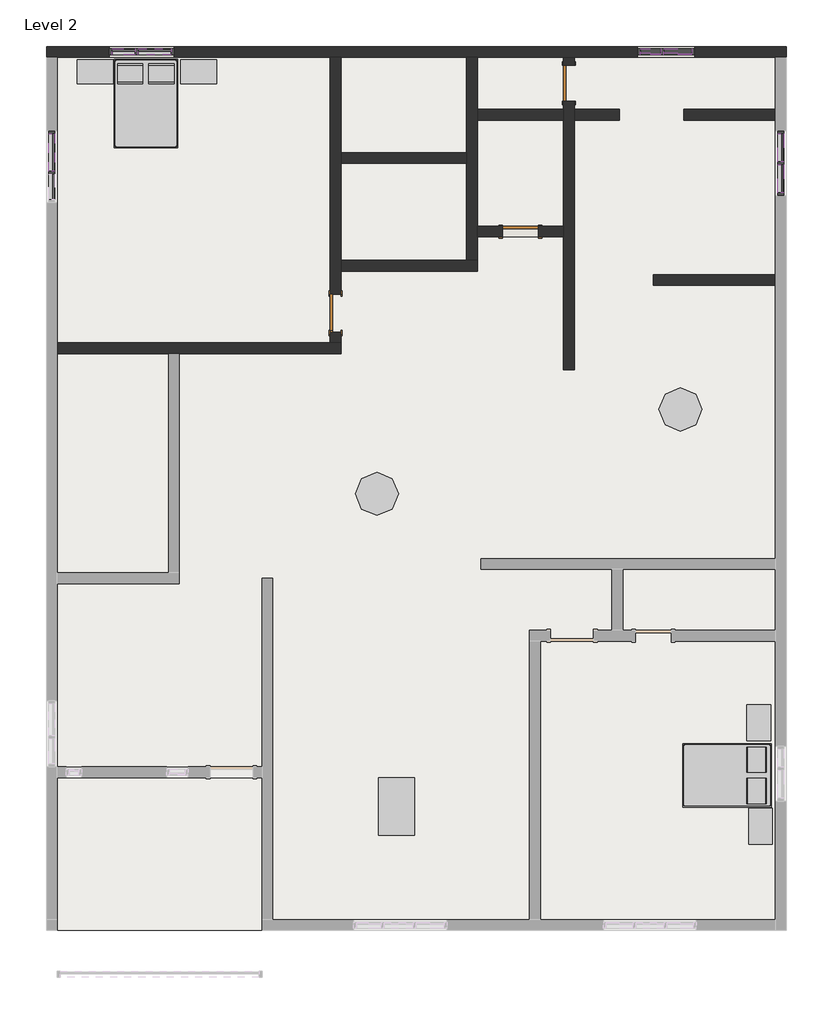
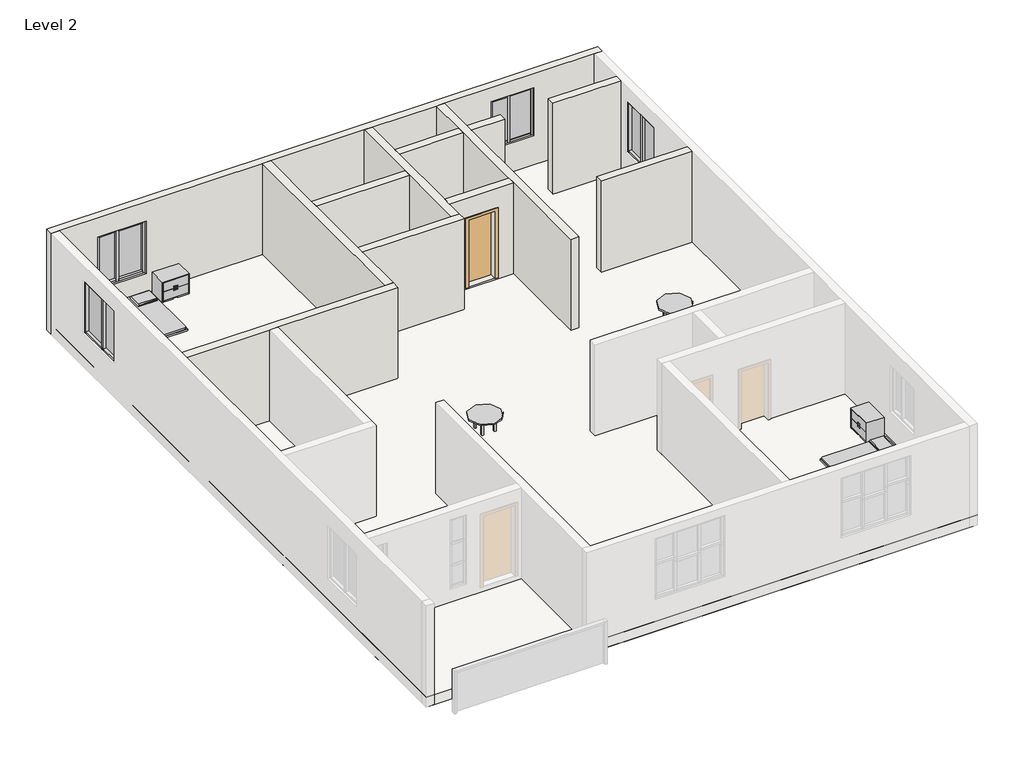
# One storey, part 3 of 3: 26 members, 12 walls, 9 furniture elements, 8 plates, 4 doors, 1 roof.
"""IFC4 building model written with IfcOpenShell, lengths in millimetres."""

from ifc_helpers import new_model, si_unit, frame, origin, place, context, project, spatial, polyline, outline, extrude, faceted_brep, transform, mapped, element, save
from components import door_a1484949, furniture_b58f7881, furniture_fb07e05e, furniture_acc2807d, furniture_52f35bf4, member_b9f3750b, member_5f1d7e17, member_e5d39754, member_104ec00a, member_3b277a63, member_6fb4a552, member_a4862887, member_e55e8fcb, member_9145ce8f, member_65d07e0b, member_13dc6413, member_cb82b20f, member_81de2198, member_b315899a, system_panel_glazed_d0271aee, system_panel_glazed_77db913b, system_panel_glazed_12bad0c7, system_panel_glazed_328f5a3b, system_panel_glazed_ae4b356e, system_panel_glazed_89fef50d, system_panel_glazed_cb6b9410

model = new_model("IFC4")

# Units and contexts
model_context = context("Model", 3, world=origin())
ifc_project = project(units=[si_unit("LENGTHUNIT", "METRE", prefix="MILLI")], contexts=[model_context])

# Site, building, storey
site = spatial("IfcSite", under=ifc_project)
building = spatial("IfcBuilding", under=site)
storey = spatial("IfcBuildingStorey", under=building, Name="Level 2", Elevation=3048.0)

# Doors
placement = place(None, origin())
door_shape = door_a1484949(model_context)
element("IfcDoor", 1, ObjectType="Single-Flush : 30\" x 80\"", at=placement, inside=storey, context=model_context, shape_type="MappedRepresentation", body=[
    mapped(door_shape, transform((-12951.6702714, 1518.6616097, 3048.0), x_axis=(0.0, 1.0, 0.0), y_axis=(-1.0, 0.0, 0.0), z_axis=(0.0, 0.0, 1.0))),
])
element("IfcDoor", 2, ObjectType="Single-Flush : 30\" x 80\"", at=placement, inside=storey, context=model_context, shape_type="MappedRepresentation", body=[
    mapped(door_shape, transform((-12951.6702714, 1480.5616097, 3048.0), x_axis=(0.0, 1.0, 0.0), y_axis=(-1.0, 0.0, 0.0), z_axis=(0.0, 0.0, 1.0))),
])
element("IfcDoor", 3, ObjectType="Single-Flush : 30\" x 80\"", at=placement, inside=storey, context=model_context, shape_type="MappedRepresentation", body=[
    mapped(door_shape, transform((-9027.3702714, 3233.1616097, 3403.6), x_axis=(1.0, 0.0, 0.0), y_axis=(0.0, 1.0, 0.0), z_axis=(0.0, 0.0, 1.0))),
])
element("IfcDoor", 4, ObjectType="Single-Flush : 30\" x 80\"", at=placement, inside=storey, context=model_context, shape_type="MappedRepresentation", body=[
    mapped(door_shape, transform((-7998.6702714, 6376.4116097, 3048.0), x_axis=(0.0, 1.0, 0.0), y_axis=(-1.0, 0.0, 0.0), z_axis=(0.0, 0.0, 1.0))),
])

# Furniture
furniture_shape = furniture_b58f7881(model_context)
element("IfcFurniture", 5, ObjectType="Bed-Box : Double 53\" x 74\"", at=placement, inside=storey, context=model_context, shape_type="MappedRepresentation", body=[
    mapped(furniture_shape, transform((-17316.7227304, 6185.3911179, 3048.0), x_axis=(1.0, 0.0, 0.0), y_axis=(0.0, 1.0, 0.0), z_axis=(0.0, 0.0, 1.0))),
])
element("IfcFurniture", 6, ObjectType="Bed-Box : Double 53\" x 74\"", at=placement, inside=storey, context=model_context, shape_type="MappedRepresentation", body=[
    mapped(furniture_shape, transform((-4411.4407632, -7959.2859313, 3048.0), x_axis=(0.0, -1.0, 0.0), y_axis=(1.0, 0.0, 0.0), z_axis=(0.0, 0.0, 1.0))),
])
furniture_2_shape = furniture_fb07e05e(model_context)
element("IfcFurniture", 7, ObjectType="Cabinet File-Lateral 3 Drawer : 30\" x 20\" x 36\"", at=placement, inside=storey, context=model_context, shape_type="MappedRepresentation", body=[
    mapped(furniture_2_shape, transform((-15679.9477575, 7558.3799858, 3048.0), x_axis=(1.0, 0.0, 0.0), y_axis=(0.0, 1.0, 0.0), z_axis=(0.0, 0.0, 1.0))),
])
element("IfcFurniture", 8, ObjectType="Cabinet File-Lateral 3 Drawer : 30\" x 20\" x 36\"", at=placement, inside=storey, context=model_context, shape_type="MappedRepresentation", body=[
    mapped(furniture_2_shape, transform((-17877.0477575, 7558.3799858, 3048.0), x_axis=(1.0, 0.0, 0.0), y_axis=(0.0, 1.0, 0.0), z_axis=(0.0, 0.0, 1.0))),
])
element("IfcFurniture", 9, ObjectType="Cabinet File-Lateral 3 Drawer : 30\" x 20\" x 36\"", at=placement, inside=storey, context=model_context, shape_type="MappedRepresentation", body=[
    mapped(furniture_2_shape, transform((-3038.4518953, -7360.8609042, 3048.0), x_axis=(0.0, -1.0, 0.0), y_axis=(1.0, 0.0, 0.0), z_axis=(0.0, 0.0, 1.0))),
])
element("IfcFurniture", 10, ObjectType="Cabinet File-Lateral 3 Drawer : 30\" x 20\" x 36\"", at=placement, inside=storey, context=model_context, shape_type="MappedRepresentation", body=[
    mapped(furniture_2_shape, transform((-3000.3518953, -9557.9609042, 3048.0), x_axis=(0.0, -1.0, 0.0), y_axis=(1.0, 0.0, 0.0), z_axis=(0.0, 0.0, 1.0))),
])
furniture_3_shape = furniture_acc2807d(model_context)
element("IfcFurniture", 11, ObjectType="Table-Coffee Rectangular : 48\" x 30\"", at=placement, inside=storey, context=model_context, shape_type="MappedRepresentation", body=[
    mapped(furniture_3_shape, transform((-11286.6594396, -9572.1720206, 3048.0), x_axis=(0.0, 1.0, 0.0), y_axis=(-1.0, 0.0, 0.0), z_axis=(0.0, 0.0, 1.0))),
])
furniture_4_shape = furniture_52f35bf4(model_context)
element("IfcFurniture", 12, ObjectType="Table-Dining Round w Chairs : 36\" Diameter", at=placement, inside=storey, context=model_context, shape_type="MappedRepresentation", body=[
    mapped(furniture_4_shape, transform((-5740.1522386, -353.8597018, 3048.0), x_axis=(1.0, 0.0, 0.0), y_axis=(0.0, 1.0, 0.0), z_axis=(0.0, 0.0, 1.0))),
])
element("IfcFurniture", 13, ObjectType="Table-Dining Round w Chairs : 36\" Diameter", at=placement, inside=storey, context=model_context, shape_type="MappedRepresentation", body=[
    mapped(furniture_4_shape, transform((-12179.0522386, -2144.5597018, 3048.0), x_axis=(1.0, 0.0, 0.0), y_axis=(0.0, 1.0, 0.0), z_axis=(0.0, 0.0, 1.0))),
])

# Members
member_shape = member_b9f3750b(model_context)
element("IfcMember", 14, ObjectType="Rectangular Mullion : 2.5\" x 5\" rectangular", at=placement, inside=storey, context=model_context, shape_type="MappedRepresentation", body=[
    mapped(member_shape, transform((-17688.7702714, 7043.1616097, 3942.1035042), x_axis=(0.0, 0.0, -1.0), y_axis=(0.0, -1.0, 0.0), z_axis=(-1.0, 0.0, 0.0))),
])
element("IfcMember", 15, ObjectType="Rectangular Mullion : 2.5\" x 5\" rectangular", at=placement, inside=storey, context=model_context, shape_type="MappedRepresentation", body=[
    mapped(member_shape, transform((-17199.8202714, 7043.1616097, 5518.94108), x_axis=(0.0, 0.0, 1.0), y_axis=(0.0, -1.0, 0.0), z_axis=(1.0, 0.0, 0.0))),
])
member_2_shape = member_5f1d7e17(model_context)
element("IfcMember", 16, ObjectType="Rectangular Mullion : 2.5\" x 5\" rectangular", at=placement, inside=storey, context=model_context, shape_type="MappedRepresentation", body=[
    mapped(member_2_shape, transform((-16444.1702714, 7043.1616097, 5518.94108), x_axis=(0.0, 0.0, 1.0), y_axis=(0.0, -1.0, 0.0), z_axis=(1.0, 0.0, 0.0))),
])
element("IfcMember", 17, ObjectType="Rectangular Mullion : 2.5\" x 5\" rectangular", at=placement, inside=storey, context=model_context, shape_type="MappedRepresentation", body=[
    mapped(member_2_shape, transform((-17136.3202714, 7043.1616097, 3942.1035042), x_axis=(0.0, 0.0, -1.0), y_axis=(0.0, -1.0, 0.0), z_axis=(-1.0, 0.0, 0.0))),
])
member_3_shape = member_e5d39754(model_context)
element("IfcMember", 18, ObjectType="Rectangular Mullion : 2.5\" x 5\" rectangular", at=placement, inside=storey, context=model_context, shape_type="MappedRepresentation", body=[
    mapped(member_3_shape, transform((-3502.8702714, 4712.7116097, 5644.9656178), x_axis=(0.0, 0.0, 1.0), y_axis=(-1.0, 0.0, 0.0), z_axis=(0.0, -1.0, 0.0))),
])
element("IfcMember", 19, ObjectType="Rectangular Mullion : 2.5\" x 5\" rectangular", at=placement, inside=storey, context=model_context, shape_type="MappedRepresentation", body=[
    mapped(member_3_shape, transform((-3502.8702714, 4058.6616097, 5644.9656178), x_axis=(0.0, 0.0, 1.0), y_axis=(-1.0, 0.0, 0.0), z_axis=(0.0, -1.0, 0.0))),
])
element("IfcMember", 20, ObjectType="Rectangular Mullion : 2.5\" x 5\" rectangular", at=placement, inside=storey, context=model_context, shape_type="MappedRepresentation", body=[
    mapped(member_3_shape, transform((-5985.7202714, 7043.1616097, 5678.8107685), x_axis=(0.0, 0.0, 1.0), y_axis=(0.0, 1.0, 0.0), z_axis=(-1.0, 0.0, 0.0))),
])
element("IfcMember", 21, ObjectType="Rectangular Mullion : 2.5\" x 5\" rectangular", at=placement, inside=storey, context=model_context, shape_type="MappedRepresentation", body=[
    mapped(member_3_shape, transform((-3502.8702714, 4649.2116097, 4078.2335743), x_axis=(0.0, 0.0, -1.0), y_axis=(-1.0, 0.0, 0.0), z_axis=(0.0, 1.0, 0.0))),
])
element("IfcMember", 22, ObjectType="Rectangular Mullion : 2.5\" x 5\" rectangular", at=placement, inside=storey, context=model_context, shape_type="MappedRepresentation", body=[
    mapped(member_3_shape, transform((-3502.8702714, 5303.2616097, 4078.2335743), x_axis=(0.0, 0.0, -1.0), y_axis=(-1.0, 0.0, 0.0), z_axis=(0.0, 1.0, 0.0))),
])
element("IfcMember", 23, ObjectType="Rectangular Mullion : 2.5\" x 5\" rectangular", at=placement, inside=storey, context=model_context, shape_type="MappedRepresentation", body=[
    mapped(member_3_shape, transform((-5395.1702714, 7043.1616097, 4231.7599798), x_axis=(0.0, 0.0, -1.0), y_axis=(0.0, 1.0, 0.0), z_axis=(1.0, 0.0, 0.0))),
])
member_4_shape = member_104ec00a(model_context)
element("IfcMember", 24, ObjectType="Rectangular Mullion : 2.5\" x 5\" rectangular", at=placement, inside=storey, context=model_context, shape_type="MappedRepresentation", body=[
    mapped(member_4_shape, transform((-3502.8702714, 4680.9616097, 4078.2335743), x_axis=(0.0, -1.0, 0.0), y_axis=(-1.0, 0.0, 0.0), z_axis=(0.0, 0.0, -1.0))),
])
member_5_shape = member_3b277a63(model_context)
element("IfcMember", 25, ObjectType="Rectangular Mullion : 2.5\" x 5\" rectangular", at=placement, inside=storey, context=model_context, shape_type="MappedRepresentation", body=[
    mapped(member_5_shape, transform((-3502.8702714, 5366.7616097, 5644.9656178), x_axis=(0.0, 1.0, 0.0), y_axis=(-1.0, 0.0, 0.0), z_axis=(0.0, 0.0, 1.0))),
])
element("IfcMember", 26, ObjectType="Rectangular Mullion : 2.5\" x 5\" rectangular", at=placement, inside=storey, context=model_context, shape_type="MappedRepresentation", body=[
    mapped(member_5_shape, transform((-3502.8702714, 3995.1616097, 4078.2335743), x_axis=(0.0, -1.0, 0.0), y_axis=(-1.0, 0.0, 0.0), z_axis=(0.0, 0.0, -1.0))),
])
member_6_shape = member_6fb4a552(model_context)
element("IfcMember", 27, ObjectType="Rectangular Mullion : 2.5\" x 5\" rectangular", at=placement, inside=storey, context=model_context, shape_type="MappedRepresentation", body=[
    mapped(member_6_shape, transform((-6487.3702714, 7043.1616097, 5678.8107685), x_axis=(0.0, 0.0, 1.0), y_axis=(0.0, 1.0, 0.0), z_axis=(-1.0, 0.0, 0.0))),
])
member_7_shape = member_a4862887(model_context)
element("IfcMember", 28, ObjectType="Rectangular Mullion : 2.5\" x 5\" rectangular", at=placement, inside=storey, context=model_context, shape_type="MappedRepresentation", body=[
    mapped(member_7_shape, transform((-6017.4702714, 7043.1616097, 4231.7599798), x_axis=(-1.0, 0.0, 0.0), y_axis=(0.0, 1.0, 0.0), z_axis=(0.0, 0.0, -1.0))),
])
element("IfcMember", 29, ObjectType="Rectangular Mullion : 2.5\" x 5\" rectangular", at=placement, inside=storey, context=model_context, shape_type="MappedRepresentation", body=[
    mapped(member_6_shape, transform((-6049.2202714, 7043.1616097, 4231.7599798), x_axis=(0.0, 0.0, -1.0), y_axis=(0.0, 1.0, 0.0), z_axis=(1.0, 0.0, 0.0))),
])
member_8_shape = member_e55e8fcb(model_context)
element("IfcMember", 30, ObjectType="Rectangular Mullion : 2.5\" x 5\" rectangular", at=placement, inside=storey, context=model_context, shape_type="MappedRepresentation", body=[
    mapped(member_8_shape, transform((-6550.8702714, 7043.1616097, 4231.7599798), x_axis=(-1.0, 0.0, 0.0), y_axis=(0.0, 1.0, 0.0), z_axis=(0.0, 0.0, -1.0))),
])
element("IfcMember", 31, ObjectType="Rectangular Mullion : 2.5\" x 5\" rectangular", at=placement, inside=storey, context=model_context, shape_type="MappedRepresentation", body=[
    mapped(member_8_shape, transform((-5331.6702714, 7043.1616097, 5678.8107685), x_axis=(1.0, 0.0, 0.0), y_axis=(0.0, 1.0, 0.0), z_axis=(0.0, 0.0, 1.0))),
])
member_9_shape = member_9145ce8f(model_context)
element("IfcMember", 32, ObjectType="Rectangular Mullion : 2.5\" x 5\" rectangular", at=placement, inside=storey, context=model_context, shape_type="MappedRepresentation", body=[
    mapped(member_9_shape, transform((-17168.0702714, 7043.1616097, 3942.1035042), x_axis=(1.0, 0.0, 0.0), y_axis=(0.0, -1.0, 0.0), z_axis=(0.0, 0.0, -1.0))),
])
member_10_shape = member_65d07e0b(model_context)
element("IfcMember", 33, ObjectType="Rectangular Mullion : 2.5\" x 5\" rectangular", at=placement, inside=storey, context=model_context, shape_type="MappedRepresentation", body=[
    mapped(member_10_shape, transform((-17752.2702714, 7043.1616097, 5518.94108), x_axis=(-1.0, 0.0, 0.0), y_axis=(0.0, -1.0, 0.0), z_axis=(0.0, 0.0, 1.0))),
])
element("IfcMember", 34, ObjectType="Rectangular Mullion : 2.5\" x 5\" rectangular", at=placement, inside=storey, context=model_context, shape_type="MappedRepresentation", body=[
    mapped(member_10_shape, transform((-16380.6702714, 7043.1616097, 3942.1035042), x_axis=(1.0, 0.0, 0.0), y_axis=(0.0, -1.0, 0.0), z_axis=(0.0, 0.0, -1.0))),
])
member_11_shape = member_13dc6413(model_context)
element("IfcMember", 35, ObjectType="Rectangular Mullion : 2.5\" x 5\" rectangular", at=placement, inside=storey, context=model_context, shape_type="MappedRepresentation", body=[
    mapped(member_11_shape, transform((-18971.4702714, 4509.5116097, 5636.3811186), x_axis=(0.0, 0.0, 1.0), y_axis=(-1.0, 0.0, 0.0), z_axis=(0.0, -1.0, 0.0))),
])
member_12_shape = member_cb82b20f(model_context)
element("IfcMember", 36, ObjectType="Rectangular Mullion : 2.5\" x 5\" rectangular", at=placement, inside=storey, context=model_context, shape_type="MappedRepresentation", body=[
    mapped(member_12_shape, transform((-18971.4702714, 4477.7616097, 4041.7365925), x_axis=(0.0, -1.0, 0.0), y_axis=(-1.0, 0.0, 0.0), z_axis=(0.0, 0.0, -1.0))),
])
member_13_shape = member_81de2198(model_context)
element("IfcMember", 37, ObjectType="Rectangular Mullion : 2.5\" x 5\" rectangular", at=placement, inside=storey, context=model_context, shape_type="MappedRepresentation", body=[
    mapped(member_13_shape, transform((-18971.4702714, 4446.0116097, 4041.7365925), x_axis=(0.0, 0.0, -1.0), y_axis=(-1.0, 0.0, 0.0), z_axis=(0.0, 1.0, 0.0))),
])
element("IfcMember", 38, ObjectType="Rectangular Mullion : 2.5\" x 5\" rectangular", at=placement, inside=storey, context=model_context, shape_type="MappedRepresentation", body=[
    mapped(member_11_shape, transform((-18971.4702714, 5303.2616097, 4041.7365925), x_axis=(0.0, 0.0, -1.0), y_axis=(-1.0, 0.0, 0.0), z_axis=(0.0, 1.0, 0.0))),
])
member_14_shape = member_b315899a(model_context)
element("IfcMember", 39, ObjectType="Rectangular Mullion : 2.5\" x 5\" rectangular", at=placement, inside=storey, context=model_context, shape_type="MappedRepresentation", body=[
    mapped(member_14_shape, transform((-18971.4702714, 5366.7616097, 5636.3811186), x_axis=(0.0, 1.0, 0.0), y_axis=(-1.0, 0.0, 0.0), z_axis=(0.0, 0.0, 1.0))),
])

# Plates
system_panel_glazed_shape = system_panel_glazed_d0271aee(model_context)
element("IfcPlate", 40, ObjectType="System Panel : Glazed", at=placement, inside=storey, context=model_context, shape_type="MappedRepresentation", body=[
    mapped(system_panel_glazed_shape, transform((-3502.8702714, 5007.9866097, 4141.7335743), x_axis=(0.0, -1.0, 0.0), y_axis=(1.0, 0.0, 0.0), z_axis=(0.0, 0.0, 1.0))),
])
element("IfcPlate", 41, ObjectType="System Panel : Glazed", at=placement, inside=storey, context=model_context, shape_type="MappedRepresentation", body=[
    mapped(system_panel_glazed_shape, transform((-3502.8702714, 4353.9366097, 4141.7335743), x_axis=(0.0, -1.0, 0.0), y_axis=(1.0, 0.0, 0.0), z_axis=(0.0, 0.0, 1.0))),
])
system_panel_glazed_2_shape = system_panel_glazed_77db913b(model_context)
element("IfcPlate", 42, ObjectType="System Panel : Glazed", at=placement, inside=storey, context=model_context, shape_type="MappedRepresentation", body=[
    mapped(system_panel_glazed_2_shape, transform((-5690.4452714, 7043.1616097, 4295.2599798), x_axis=(-1.0, 0.0, 0.0), y_axis=(0.0, -1.0, 0.0), z_axis=(0.0, 0.0, 1.0))),
])
system_panel_glazed_3_shape = system_panel_glazed_12bad0c7(model_context)
element("IfcPlate", 43, ObjectType="System Panel : Glazed", at=placement, inside=storey, context=model_context, shape_type="MappedRepresentation", body=[
    mapped(system_panel_glazed_3_shape, transform((-6268.2952714, 7043.1616097, 4295.2599798), x_axis=(-1.0, 0.0, 0.0), y_axis=(0.0, -1.0, 0.0), z_axis=(0.0, 0.0, 1.0))),
])
system_panel_glazed_4_shape = system_panel_glazed_328f5a3b(model_context)
element("IfcPlate", 44, ObjectType="System Panel : Glazed", at=placement, inside=storey, context=model_context, shape_type="MappedRepresentation", body=[
    mapped(system_panel_glazed_4_shape, transform((-17444.2952714, 7043.1616097, 4005.6035042), x_axis=(1.0, 0.0, 0.0), y_axis=(0.0, 1.0, 0.0), z_axis=(0.0, 0.0, 1.0))),
])
system_panel_glazed_5_shape = system_panel_glazed_ae4b356e(model_context)
element("IfcPlate", 45, ObjectType="System Panel : Glazed", at=placement, inside=storey, context=model_context, shape_type="MappedRepresentation", body=[
    mapped(system_panel_glazed_5_shape, transform((-16790.2452714, 7043.1616097, 4005.6035042), x_axis=(1.0, 0.0, 0.0), y_axis=(0.0, 1.0, 0.0), z_axis=(0.0, 0.0, 1.0))),
])
system_panel_glazed_6_shape = system_panel_glazed_89fef50d(model_context)
element("IfcPlate", 46, ObjectType="System Panel : Glazed", at=placement, inside=storey, context=model_context, shape_type="MappedRepresentation", body=[
    mapped(system_panel_glazed_6_shape, transform((-18971.4702714, 4906.3866097, 4105.2365925), x_axis=(0.0, -1.0, 0.0), y_axis=(1.0, 0.0, 0.0), z_axis=(0.0, 0.0, 1.0))),
])
system_panel_glazed_7_shape = system_panel_glazed_cb6b9410(model_context)
element("IfcPlate", 47, ObjectType="System Panel : Glazed", at=placement, inside=storey, context=model_context, shape_type="MappedRepresentation", body=[
    mapped(system_panel_glazed_7_shape, transform((-18971.4702714, 4176.1366097, 4105.2365925), x_axis=(0.0, -1.0, 0.0), y_axis=(1.0, 0.0, 0.0), z_axis=(0.0, 0.0, 1.0))),
])

# Roof
element("IfcRoof", 48, ObjectType="Generic - 12\"", at=placement, inside=storey, context=model_context, shape_type="SweptSolid", body=[
    extrude(outline(polyline([(-19085.7702714, 7157.4616097), (-3388.5702714, 7157.4616097), (-3388.5702714, -11587.7383903), (-19085.7702714, -11587.7383903), (-19085.7702714, 7157.4616097)])), frame((0.0, 0.0, 3048.0), z_axis=(0.0, 0.0, 1.0), x_axis=(1.0, 0.0, 0.0)), (0.0, 0.0, 1.0), 304.8),
])

# Walls
element("IfcWall", 49, ObjectType="9\"", at=placement, inside=storey, context=model_context, shape_type="Brep", body=[
    faceted_brep([(-19085.7702714, 6928.8616097, 3048.0), (-18857.1702714, 6928.8616097, 3048.0), (-13065.9702714, 6928.8616097, 3048.0), (-12837.3702714, 6928.8616097, 3048.0), (-10170.3702714, 6928.8616097, 3048.0), (-9941.7702714, 6928.8616097, 3048.0), (-8112.9702714, 6928.8616097, 3048.0), (-7884.3702714, 6928.8616097, 3048.0), (-3617.1702714, 6928.8616097, 3048.0), (-3388.5702714, 6928.8616097, 3048.0), (-3388.5702714, 6928.8616097, 6096.0), (-3617.1702714, 6928.8616097, 6096.0), (-7884.3702714, 6928.8616097, 6096.0), (-8112.9702714, 6928.8616097, 6096.0), (-9941.7702714, 6928.8616097, 6096.0), (-10170.3702714, 6928.8616097, 6096.0), (-12837.3702714, 6928.8616097, 6096.0), (-13065.9702714, 6928.8616097, 6096.0), (-18857.1702714, 6928.8616097, 6096.0), (-19085.7702714, 6928.8616097, 6096.0), (-5331.6702714, 6928.8616097, 5678.8107685), (-5331.6702714, 6928.8616097, 4231.7599798), (-6550.8702714, 6928.8616097, 4231.7599798), (-6550.8702714, 6928.8616097, 5678.8107685), (-17752.2702714, 6928.8616097, 3942.1035042), (-17752.2702714, 6928.8616097, 5518.94108), (-16380.6702714, 6928.8616097, 5518.94108), (-16380.6702714, 6928.8616097, 3942.1035042), (-3388.5702714, 7157.4616097, 3048.0), (-19085.7702714, 7157.4616097, 3048.0), (-19085.7702714, 7157.4616097, 6096.0), (-3388.5702714, 7157.4616097, 6096.0), (-5331.6702714, 7157.4616097, 4231.7599798), (-5331.6702714, 7157.4616097, 5678.8107685), (-6550.8702714, 7157.4616097, 5678.8107685), (-6550.8702714, 7157.4616097, 4231.7599798), (-17752.2702714, 7157.4616097, 5518.94108), (-17752.2702714, 7157.4616097, 3942.1035042), (-16380.6702714, 7157.4616097, 3942.1035042), (-16380.6702714, 7157.4616097, 5518.94108)], [[[0, 1, 2, 3, 4, 5, 6, 7, 8, 9, 10, 11, 12, 13, 14, 15, 16, 17, 18, 19], [20, 21, 22, 23], [24, 25, 26, 27]], [[28, 29, 30, 31], [32, 33, 34, 35], [36, 37, 38, 39]], [[9, 8, 7, 6, 5, 4, 3, 2, 1, 0, 29, 28]], [[19, 18, 17, 16, 15, 14, 13, 12, 11, 10, 31, 30]], [[10, 9, 28, 31]], [[0, 19, 30, 29]], [[32, 21, 20, 33]], [[33, 20, 23, 34]], [[34, 23, 22, 35]], [[21, 32, 35, 22]], [[36, 25, 24, 37]], [[25, 36, 39, 26]], [[26, 39, 38, 27]], [[37, 24, 27, 38]]]),
])
element("IfcWall", 50, ObjectType="9\"", at=placement, inside=storey, context=model_context, shape_type="Brep", body=[
    faceted_brep([(-12837.3702714, 870.9616097, 3048.0), (-13065.9702714, 870.9616097, 3048.0), (-18857.1702714, 870.9616097, 3048.0), (-18857.1702714, 870.9616097, 6096.0), (-13065.9702714, 870.9616097, 6096.0), (-12837.3702714, 870.9616097, 6096.0), (-12837.3702714, 642.3616097, 3048.0), (-12837.3702714, 642.3616097, 6096.0), (-16266.3702714, 642.3616097, 6096.0), (-16494.9702714, 642.3616097, 6096.0), (-18857.1702714, 642.3616097, 6096.0), (-18857.1702714, 642.3616097, 3048.0), (-16494.9702714, 642.3616097, 3048.0), (-16266.3702714, 642.3616097, 3048.0)], [[[0, 1, 2, 3, 4, 5]], [[6, 7, 8, 9, 10, 11, 12, 13]], [[2, 1, 0, 6, 13, 12, 11]], [[5, 4, 3, 10, 9, 8, 7]], [[3, 2, 11, 10]], [[0, 5, 7, 6]]]),
])
element("IfcWall", 51, ObjectType="9\"", at=placement, inside=storey, context=model_context, shape_type="Brep", body=[
    faceted_brep([(-12837.3702714, 6928.8616097, 6096.0), (-12837.3702714, 4909.5616097, 6096.0), (-12837.3702714, 4680.9616097, 6096.0), (-12837.3702714, 2623.5616097, 6096.0), (-12837.3702714, 2394.9616097, 6096.0), (-12837.3702714, 870.9616097, 6096.0), (-12837.3702714, 870.9616097, 3048.0), (-12837.3702714, 1099.5616097, 3048.0), (-12837.3702714, 1099.5616097, 5080.0), (-12837.3702714, 1899.6616097, 5080.0), (-12837.3702714, 1899.6616097, 3048.0), (-12837.3702714, 2394.9616097, 3048.0), (-12837.3702714, 2623.5616097, 3048.0), (-12837.3702714, 4680.9616097, 3048.0), (-12837.3702714, 4909.5616097, 3048.0), (-12837.3702714, 6928.8616097, 3048.0), (-13065.9702714, 870.9616097, 6096.0), (-13065.9702714, 6928.8616097, 6096.0), (-13065.9702714, 6928.8616097, 3048.0), (-13065.9702714, 1899.6616097, 3048.0), (-13065.9702714, 1899.6616097, 5080.0), (-13065.9702714, 1099.5616097, 5080.0), (-13065.9702714, 1099.5616097, 3048.0), (-13065.9702714, 870.9616097, 3048.0)], [[[0, 1, 2, 3, 4, 5, 6, 7, 8, 9, 10, 11, 12, 13, 14, 15]], [[16, 17, 18, 19, 20, 21, 22, 23]], [[6, 23, 22, 7]], [[18, 15, 14, 13, 12, 11, 10, 19]], [[5, 4, 3, 2, 1, 0, 17, 16]], [[6, 5, 16, 23]], [[0, 15, 18, 17]], [[20, 19, 10, 9]], [[20, 9, 8, 21]], [[21, 8, 7, 22]]]),
])
element("IfcWall", 52, ObjectType="9\"", at=placement, inside=storey, context=model_context, shape_type="Brep", body=[
    faceted_brep([(-12837.3702714, 2394.9616097, 3048.0), (-9941.7702714, 2394.9616097, 3048.0), (-9941.7702714, 2394.9616097, 6096.0), (-12837.3702714, 2394.9616097, 6096.0), (-12837.3702714, 2623.5616097, 3048.0), (-12837.3702714, 2623.5616097, 6096.0), (-10170.3702714, 2623.5616097, 6096.0), (-9941.7702714, 2623.5616097, 6096.0), (-9941.7702714, 2623.5616097, 3048.0), (-10170.3702714, 2623.5616097, 3048.0)], [[[0, 1, 2, 3]], [[4, 5, 6, 7, 8, 9]], [[1, 0, 4, 9, 8]], [[3, 2, 7, 6, 5]], [[0, 3, 5, 4]], [[2, 1, 8, 7]]]),
])
element("IfcWall", 53, ObjectType="9\"", at=placement, inside=storey, context=model_context, shape_type="Brep", body=[
    faceted_brep([(-9941.7702714, 2623.5616097, 3048.0), (-9941.7702714, 3118.8616097, 3048.0), (-9941.7702714, 3347.4616097, 3048.0), (-9941.7702714, 5595.3616097, 3048.0), (-9941.7702714, 5823.9616097, 3048.0), (-9941.7702714, 6928.8616097, 3048.0), (-9941.7702714, 6928.8616097, 6096.0), (-9941.7702714, 5823.9616097, 6096.0), (-9941.7702714, 5595.3616097, 6096.0), (-9941.7702714, 3347.4616097, 6096.0), (-9941.7702714, 3118.8616097, 6096.0), (-9941.7702714, 2623.5616097, 6096.0), (-10170.3702714, 2623.5616097, 3048.0), (-10170.3702714, 2623.5616097, 6096.0), (-10170.3702714, 4680.9616097, 6096.0), (-10170.3702714, 4909.5616097, 6096.0), (-10170.3702714, 6928.8616097, 6096.0), (-10170.3702714, 6928.8616097, 3048.0), (-10170.3702714, 4909.5616097, 3048.0), (-10170.3702714, 4680.9616097, 3048.0)], [[[0, 1, 2, 3, 4, 5, 6, 7, 8, 9, 10, 11]], [[12, 13, 14, 15, 16, 17, 18, 19]], [[5, 4, 3, 2, 1, 0, 12, 19, 18, 17]], [[11, 10, 9, 8, 7, 6, 16, 15, 14, 13]], [[0, 11, 13, 12]], [[6, 5, 17, 16]]]),
])
element("IfcWall", 54, ObjectType="9\"", at=placement, inside=storey, context=model_context, shape_type="SweptSolid", body=[
    extrude(outline(polyline([(-10170.3702714, 4680.9616097), (-12837.3702714, 4680.9616097), (-12837.3702714, 4909.5616097), (-10170.3702714, 4909.5616097), (-10170.3702714, 4680.9616097)])), frame((0.0, 0.0, 3048.0), z_axis=(0.0, 0.0, 1.0), x_axis=(1.0, 0.0, 0.0)), (0.0, 0.0, 1.0), 3048.0),
])
element("IfcWall", 55, ObjectType="9\"", at=placement, inside=storey, context=model_context, shape_type="Brep", body=[
    faceted_brep([(-8112.9702714, 6928.8616097, 3048.0), (-8112.9702714, 6757.4116097, 3048.0), (-8112.9702714, 6757.4116097, 5080.0), (-8112.9702714, 5995.4116097, 5080.0), (-8112.9702714, 5995.4116097, 3048.0), (-8112.9702714, 5823.9616097, 3048.0), (-8112.9702714, 5595.3616097, 3048.0), (-8112.9702714, 3347.4616097, 3048.0), (-8112.9702714, 3118.8616097, 3048.0), (-8112.9702714, 299.4616097, 3048.0), (-8112.9702714, 299.4616097, 6096.0), (-8112.9702714, 3118.8616097, 6096.0), (-8112.9702714, 3347.4616097, 6096.0), (-8112.9702714, 5595.3616097, 6096.0), (-8112.9702714, 5823.9616097, 6096.0), (-8112.9702714, 6928.8616097, 6096.0), (-7884.3702714, 6757.4116097, 5080.0), (-7884.3702714, 6757.4116097, 3048.0), (-7884.3702714, 6928.8616097, 3048.0), (-7884.3702714, 6928.8616097, 6096.0), (-7884.3702714, 5823.9616097, 6096.0), (-7884.3702714, 5595.3616097, 6096.0), (-7884.3702714, 299.4616097, 6096.0), (-7884.3702714, 299.4616097, 3048.0), (-7884.3702714, 5595.3616097, 3048.0), (-7884.3702714, 5823.9616097, 3048.0), (-7884.3702714, 5995.4116097, 3048.0), (-7884.3702714, 5995.4116097, 5080.0)], [[[0, 1, 2, 3, 4, 5, 6, 7, 8, 9, 10, 11, 12, 13, 14, 15]], [[16, 17, 18, 19, 20, 21, 22, 23, 24, 25, 26, 27]], [[18, 17, 1, 0]], [[26, 25, 24, 23, 9, 8, 7, 6, 5, 4]], [[10, 9, 23, 22]], [[15, 14, 13, 12, 11, 10, 22, 21, 20, 19]], [[0, 15, 19, 18]], [[2, 1, 17, 16]], [[3, 2, 16, 27]], [[4, 3, 27, 26]]]),
])
element("IfcWall", 56, ObjectType="9\"", at=placement, inside=storey, context=model_context, shape_type="SweptSolid", body=[
    extrude(outline(polyline([(-8112.9702714, 5595.3616097), (-9941.7702714, 5595.3616097), (-9941.7702714, 5823.9616097), (-8112.9702714, 5823.9616097), (-8112.9702714, 5595.3616097)])), frame((0.0, 0.0, 3048.0), z_axis=(0.0, 0.0, 1.0), x_axis=(1.0, 0.0, 0.0)), (0.0, 0.0, 1.0), 3048.0),
])
element("IfcWall", 57, ObjectType="9\"", at=placement, inside=storey, context=model_context, shape_type="SweptSolid", body=[
    extrude(outline(polyline([(3048.0, -9941.7702714), (3048.0, -8112.9702714), (6096.0, -8112.9702714), (6096.0, -9941.7702714), (3048.0, -9941.7702714)]), holes=[polyline([(3403.6, -9408.3702714), (5435.6, -9408.3702714), (5435.6, -8646.3702714), (3403.6, -8646.3702714), (3403.6, -9408.3702714)])]), frame((0.0, 3118.8616097, 0.0), z_axis=(0.0, 1.0, 0.0), x_axis=(0.0, 0.0, 1.0)), (0.0, 0.0, 1.0), 228.6),
])
element("IfcWall", 58, ObjectType="9\"", at=placement, inside=storey, context=model_context, shape_type="SweptSolid", body=[
    extrude(outline(polyline([(-6931.8702714, 5595.3616097), (-7884.3702714, 5595.3616097), (-7884.3702714, 5823.9616097), (-6931.8702714, 5823.9616097), (-6931.8702714, 5595.3616097)])), frame((0.0, 0.0, 3048.0), z_axis=(0.0, 0.0, 1.0), x_axis=(1.0, 0.0, 0.0)), (0.0, 0.0, 1.0), 3048.0),
])
element("IfcWall", 59, ObjectType="9\"", at=placement, inside=storey, context=model_context, shape_type="SweptSolid", body=[
    extrude(outline(polyline([(-5560.2702714, 5823.9616097), (-3617.1702714, 5823.9616097), (-3617.1702714, 5595.3616097), (-5560.2702714, 5595.3616097), (-5560.2702714, 5823.9616097)])), frame((0.0, 0.0, 3048.0), z_axis=(0.0, 0.0, 1.0), x_axis=(1.0, 0.0, 0.0)), (0.0, 0.0, 1.0), 3048.0),
])
element("IfcWall", 60, ObjectType="9\"", at=placement, inside=storey, context=model_context, shape_type="SweptSolid", body=[
    extrude(outline(polyline([(-6207.9702714, 2318.7616097), (-3617.1702714, 2318.7616097), (-3617.1702714, 2090.1616097), (-6207.9702714, 2090.1616097), (-6207.9702714, 2318.7616097)])), frame((0.0, 0.0, 3048.0), z_axis=(0.0, 0.0, 1.0), x_axis=(1.0, 0.0, 0.0)), (0.0, 0.0, 1.0), 3048.0),
])

save(model, "model.ifc")

# Revit data of these elements
# Type "Single-Flush : 30\" x 80\""
#   Type Mark = "5"
#   Construction Type Id = "MDOOR"
#   Assembly Code = "C1020"
#   Analytic Construction = "Metal"
#   Thickness = 0' - 2"
#   Heat Transfer Coefficient (U) = 0.651978 BTU/(h·ft²·°F)
#   Height = 6' - 8"
#   Trim Projection Ext = 0' - 1"
#   Trim Projection Int = 0' - 1"
#   Trim Width = 0' - 3"
#   Width = 2' - 6"
#   Define Thermal Properties by = 1
#   Define Thermal Properties by = 1
#   Door Material = Door - Panel
#   Frame Material = Door - Frame
#   Visual Light Transmittance = 0
#   Solar Heat Gain Coefficient = 0
#   Function = (empty or 0)
#   Wall Closure = (empty or 0)
# Type "Bed-Box : Double 53\" x 74\""
#   Assembly Code = "E2020200"
#   Length = 6' - 2"
#   Width = 4' - 5"
#   Frame Material = Birch
#   Mattress Material = Linen, White
#   Default Elevation = 0
# Type "Cabinet File-Lateral 3 Drawer : 30\" x 20\" x 36\""
#   Assembly Code = "E2020200"
#   Depth = 1' - 8"
#   Height = 3' - 0"
#   Width = 2' - 6"
#   Material = Metal - Steel
#   Default Elevation = 0
# Type "Table-Coffee Rectangular : 48\" x 30\""
#   Assembly Code = "E2020200"
#   Height = 1' - 1"
#   Length = 4' - 0"
#   Width = 2' - 6"
#   Base Material = Metal - Chrome
#   Table Top Material = Glass - Clear, Grey
#   Default Elevation = 0
# Type "Table-Dining Round w Chairs : 36\" Diameter"
#   Assembly Code = "E2020200"
#   Radius = 1' - 6"
#   Diameter = 3' - 0"
#   Height = 2' - 6"
#   Chairs = 4
#   Base Material = Pine
#   Top Material = Laminate, Linen, Matte
#   Default Elevation = 0
# Type "Rectangular Mullion : 2.5\" x 5\" rectangular"
#   built-in parameter 1007304 = 0.416667 (stored number, unit not read)
#   built-in parameter 1007301 = 0.104167 (stored number, unit not read)
#   built-in parameter 1007300 = 0.104167 (stored number, unit not read)
# Type "System Panel : Glazed"
#   Construction Type Id = "GSP4R"
#   Analytic Construction = "1/8 in Pilkington single glazing"
#   Visual Light Transmittance = 0.9
#   Solar Heat Gain Coefficient = 0.86
#   Heat Transfer Coefficient (U) = 1.18115 BTU/(h·ft²·°F)
#   Define Thermal Properties by = 1
# Type "Generic - 12\""
#   Assembly Code = "B1020"
#   Layers, outside or top first: 1' - 0" no material (function 1)
# Type "9\""
#   Assembly Code = "B2010"
#   Layers, outside or top first: 0' - 9" no material (function 1)
# Elements 1, 2, 3, 4 (IfcDoor, "Single-Flush : 30\" x 80\"")
#   Phase Created = New Construction
#   Materials on its faces: "Door - Frame", "Door - Panel"
# Elements 5, 6 (IfcFurniture, "Bed-Box : Double 53\" x 74\"")
#   Phase Created = New Construction
#   Materials on its faces: "Birch", "Linen, White"
# Elements 7, 8, 9, 10 (IfcFurniture, "Cabinet File-Lateral 3 Drawer : 30\" x 20\" x 36\"")
#   Phase Created = New Construction
#   Materials on its faces: "Metal - Steel"
# Element 11 (IfcFurniture, "Table-Coffee Rectangular : 48\" x 30\"")
#   Phase Created = New Construction
#   Materials on its faces: "Metal - Chrome", "Glass - Clear, Grey"
# Elements 12, 13 (IfcFurniture, "Table-Dining Round w Chairs : 36\" Diameter")
#   Phase Created = New Construction
#   Materials on its faces: "Pine", "Laminate, Linen, Matte"
# Elements 14, 15, 16, 17, 18, 19, 20, 21, 22, 23, 24, 25, 26, 27, 28, 29, 30, 31, 32, 33, 34, 35, 36, 37, 38, 39 (IfcMember, "Rectangular Mullion : 2.5\" x 5\" rectangular")
#   Phase Created = New Construction
#   Materials on its faces: "Aluminum"
# Elements 40, 41, 42, 43, 44, 45, 46, 47 (IfcPlate, "System Panel : Glazed")
#   Phase Created = New Construction
#   Materials on its faces: "Glass"
# Element 48 (IfcRoof, "Generic - 12\"")
#   built-in parameter 1001705 = 11 (stored number, unit not read)
#   built-in parameter 1001710 = 33615
#   Phase Created = New Construction
#   Materials on its faces: "Default Roof"
# Elements 49, 50, 51, 52, 53, 54, 55, 56, 57, 58, 59, 60 (IfcWall, "9\"")
#   Top Offset = 0' - 0"
#   Base Offset = 0' - 0"
#   Unconnected Height = 10' - 0"
#   wall height = 10' - 0"
#   Phase Created = New Construction
#   Base Constraint = Level 2
#   Materials on its faces: "Default Wall"
# Materials
#   "Door - Panel": class "Wood", colour RGB 210 159 95, transparency 0, Cost = 0
#   "Door - Frame": colour RGB 118 70 51, transparency 0, Cost = 0
#   "Birch": class "Wood", colour RGB 224 178 126, transparency 0, Description = "Betula Alleghaniensis", Cost = 0
#   "Linen, White": class "Textile", colour RGB 247 247 239, transparency 0, Description = "Linen, white", Cost = 0
#   "Metal - Steel": colour RGB 209 209 209, transparency 0
#   "Metal - Chrome": colour RGB 57 57 57, transparency 0
#   "Glass - Clear, Grey": colour RGB 252 255 255, transparency 0.64
#   "Pine": class "Wood", colour RGB 223 192 134, transparency 0, Description = "Pinus Echinata", Cost = 0
#   "Laminate, Linen, Matte": class "Plastic", colour RGB 249 239 230, transparency 0, Description = "Plastic Laminate - Linen, Matte", Cost = 0
#   "Aluminum": class "Metal", colour RGB 247 247 247, transparency 0, Description = "Aluminum 6061", Cost = 0
#   "Glass": class "Glass", colour RGB 0 128 192, transparency 0.75, Description = "Soda Lime Glass", Cost = 0
#   "Default Roof": colour RGB 88 101 114, transparency 0, Cost = 0
#   "Default Wall": colour RGB 128 128 128, transparency 0, Cost = 0
